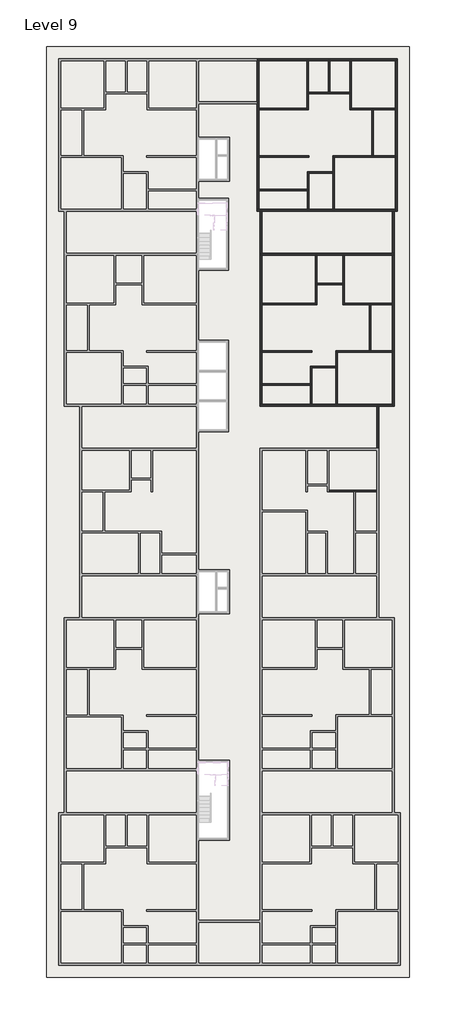
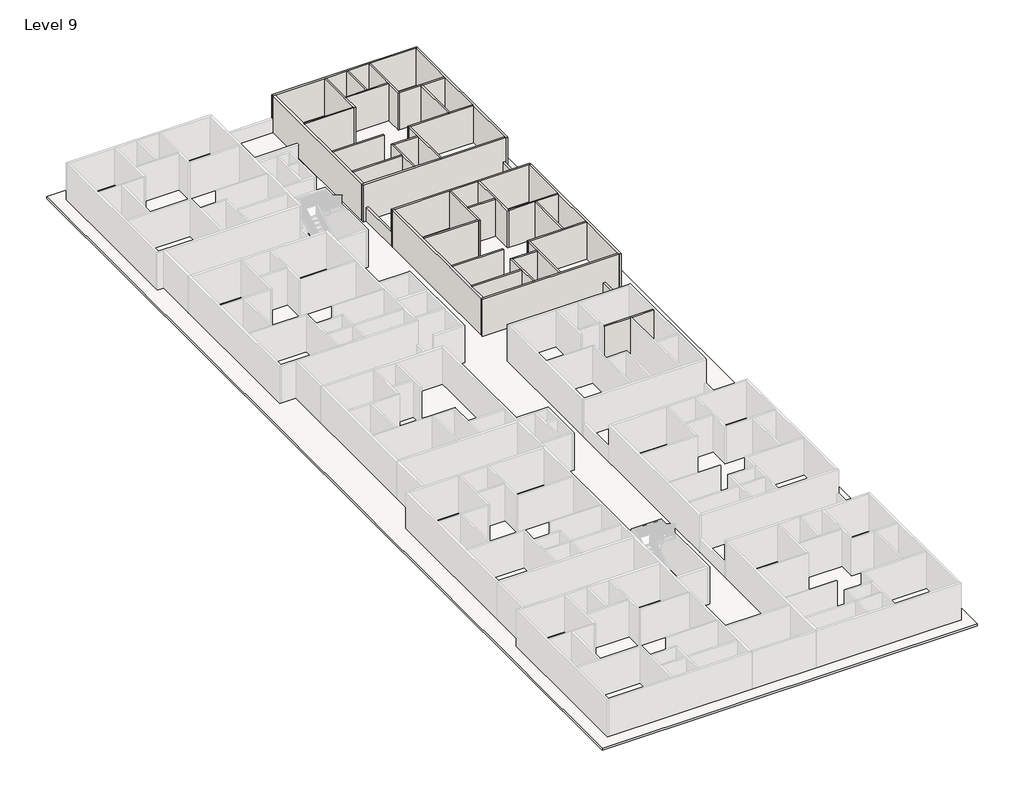
# One storey, part 4 of 8: 37 walls, 1 roof, 1 slab.
"""IFC4 building model written with IfcOpenShell, lengths in millimetres."""

from ifc_helpers import new_model, si_unit, frame, origin, place, context, project, spatial, polyline, outline, extrude, faceted_brep, element, save

model = new_model("IFC4")

# Units and contexts
model_context = context("Model", 3, world=origin())
ifc_project = project(units=[si_unit("LENGTHUNIT", "METRE", prefix="MILLI")], contexts=[model_context])

# Site, building, storey
site = spatial("IfcSite", under=ifc_project)
building = spatial("IfcBuilding", under=site)
storey = spatial("IfcBuildingStorey", under=building, Name="Level 9", Elevation=49618.6172466)

# Roof
placement = place(None, origin())
element("IfcRoof", 1, ObjectType="SLAB", at=placement, inside=storey, context=model_context, shape_type="SweptSolid", body=[
    extrude(outline(polyline([(-15237.9415084, -35021.5344126), (-15237.9415084, 36097.9216096), (12498.9443719, 36097.9216096), (12498.9443719, -35021.5344126), (-15237.9415084, -35021.5344126)]), holes=[polyline([(-3617.4415084, 29152.4900967), (-3617.4415084, 25799.6900967), (-1255.2415084, 25799.6900967), (-1255.2415084, 29152.4900967), (-3617.4415084, 29152.4900967)]), polyline([(-3617.4415084, 24490.1216096), (-3617.4415084, 19003.7216096), (-1331.4415084, 19003.7216096), (-1331.4415084, 24490.1216096), (-3617.4415084, 24490.1216096)]), polyline([(-3617.4415084, 13669.6303368), (-3617.4415084, 6659.2303368), (-1331.4415084, 6659.2303368), (-1331.4415084, 13669.6303368), (-3617.4415084, 13669.6303368)]), polyline([(-3617.4415084, -3882.2751812), (-3617.4415084, -7235.0751812), (-1255.2415084, -7235.0751812), (-1255.2415084, -3882.2751812), (-3617.4415084, -3882.2751812)]), polyline([(-3617.4415084, -18429.9851539), (-3617.4415084, -24525.9851539), (-1229.8415084, -24525.9851539), (-1229.8415084, -18429.9851539), (-3617.4415084, -18429.9851539)])]), frame((0.0, 0.0, 49618.6172466), z_axis=(0.0, 0.0, 1.0), x_axis=(1.0, 0.0, 0.0)), (0.0, 0.0, 1.0), 152.4),
])

# Slab
element("IfcSlab", 2, ObjectType="FLOOR", at=placement, inside=storey, context=model_context, shape_type="SweptSolid", body=[
    extrude(outline(polyline([(-14323.5415084, 35183.5216096), (11584.5443719, 35183.5216096), (11584.5443719, 23499.5216096), (11360.9214687, 23499.5216096), (11360.9214687, 8615.1216096), (10173.4714687, 8615.1216096), (10173.4714687, -7538.7344126), (11360.9214687, -7538.7344126), (11360.9214687, -22423.1344126), (11813.0584916, -22423.1344126), (11813.0584916, -34107.1344126), (11584.5443719, -34107.1344126), (-14323.5415084, -34107.1344126), (-14323.5415084, 35183.5216096)]), holes=[polyline([(-3617.4415084, 29152.4900967), (-3617.4415084, 25799.6900967), (-1255.2415084, 25799.6900967), (-1255.2415084, 29152.4900967), (-3617.4415084, 29152.4900967)]), polyline([(-3617.4415084, 24490.1216096), (-3617.4415084, 19003.7216096), (-1331.4415084, 19003.7216096), (-1331.4415084, 24490.1216096), (-3617.4415084, 24490.1216096)]), polyline([(-3617.4415084, 13669.6303368), (-3617.4415084, 6659.2303368), (-1331.4415084, 6659.2303368), (-1331.4415084, 13669.6303368), (-3617.4415084, 13669.6303368)]), polyline([(-3617.4415084, -3882.2751812), (-3617.4415084, -7235.0751812), (-1255.2415084, -7235.0751812), (-1255.2415084, -3882.2751812), (-3617.4415084, -3882.2751812)]), polyline([(-3617.4415084, -18429.9851539), (-3617.4415084, -24525.9851539), (-1229.8415084, -24525.9851539), (-1229.8415084, -18429.9851539), (-3617.4415084, -18429.9851539)])]), frame((0.0, 0.0, 49009.0172466), z_axis=(0.0, 0.0, 1.0), x_axis=(1.0, 0.0, 0.0)), (0.0, 0.0, 1.0), 609.6),
])

# Walls
element("IfcWall", 3, ObjectType="4.5\"", at=placement, inside=storey, context=model_context, shape_type="Brep", body=[
    faceted_brep([(6363.4714687, 2100.0216096, 49618.6172466), (8282.4584916, 2100.0216096, 49618.6172466), (8396.7584916, 2100.0216096, 49618.6172466), (10021.0714687, 2100.0216096, 49618.6172466), (10021.0714687, 2100.0216096, 52666.6172466), (8396.7584916, 2100.0216096, 52666.6172466), (8282.4584916, 2100.0216096, 52666.6172466), (6363.4714687, 2100.0216096, 52666.6172466), (6363.4714687, 2214.3216096, 49618.6172466), (6363.4714687, 2214.3216096, 52666.6172466), (10021.0714687, 2214.3216096, 52666.6172466), (10021.0714687, 2214.3216096, 49618.6172466)], [[[0, 1, 2, 3, 4, 5, 6, 7]], [[8, 9, 10, 11]], [[3, 2, 1, 0, 8, 11]], [[0, 7, 9, 8]], [[4, 3, 11, 10]], [[7, 6, 5, 4, 10, 9]]]),
])
element("IfcWall", 4, ObjectType="4.5\"", at=placement, inside=storey, context=model_context, shape_type="Brep", body=[
    faceted_brep([(5315.7214687, 20146.7216096, 49618.6172466), (5315.7214687, 16489.1216096, 49618.6172466), (5315.7214687, 16374.8216096, 49618.6172466), (5315.7214687, 16374.8216096, 52666.6172466), (5315.7214687, 16489.1216096, 52666.6172466), (5315.7214687, 20146.7216096, 52666.6172466), (5430.0214687, 20146.7216096, 49618.6172466), (5430.0214687, 20146.7216096, 52666.6172466), (5430.0214687, 18013.1216096, 52666.6172466), (5430.0214687, 17898.8216096, 52666.6172466), (5430.0214687, 16374.8216096, 52666.6172466), (5430.0214687, 16374.8216096, 49618.6172466), (5430.0214687, 17898.8216096, 49618.6172466), (5430.0214687, 18013.1216096, 49618.6172466)], [[[0, 1, 2, 3, 4, 5]], [[6, 7, 8, 9, 10, 11, 12, 13]], [[2, 1, 0, 6, 13, 12, 11]], [[0, 5, 7, 6]], [[3, 2, 11, 10]], [[5, 4, 3, 10, 9, 8, 7]]]),
])
element("IfcWall", 5, ObjectType="4.5\"", at=placement, inside=storey, context=model_context, shape_type="SweptSolid", body=[
    extrude(outline(polyline([(1259.3584916, 16489.1216096), (5315.7214687, 16489.1216096), (5315.7214687, 16374.8216096), (1259.3584916, 16374.8216096), (1259.3584916, 16489.1216096)])), frame((0.0, 0.0, 49618.6172466), z_axis=(0.0, 0.0, 1.0), x_axis=(1.0, 0.0, 0.0)), (0.0, 0.0, 1.0), 3048.0),
])
element("IfcWall", 6, ObjectType="4.5\"", at=placement, inside=storey, context=model_context, shape_type="SweptSolid", body=[
    extrude(outline(polyline([(7436.6214687, 17898.8216096), (5430.0214687, 17898.8216096), (5430.0214687, 18013.1216096), (7436.6214687, 18013.1216096), (7436.6214687, 17898.8216096)])), frame((0.0, 0.0, 49618.6172466), z_axis=(0.0, 0.0, 1.0), x_axis=(1.0, 0.0, 0.0)), (0.0, 0.0, 1.0), 3048.0),
])
element("IfcWall", 7, ObjectType="4.5\"", at=placement, inside=storey, context=model_context, shape_type="Brep", body=[
    faceted_brep([(7436.6214687, 20146.7216096, 49618.6172466), (7436.6214687, 18013.1216096, 49618.6172466), (7436.6214687, 17898.8216096, 49618.6172466), (7436.6214687, 16374.8216096, 49618.6172466), (7436.6214687, 16374.8216096, 52666.6172466), (7436.6214687, 17898.8216096, 52666.6172466), (7436.6214687, 18013.1216096, 52666.6172466), (7436.6214687, 20146.7216096, 52666.6172466), (7550.9214687, 20146.7216096, 49618.6172466), (7550.9214687, 20146.7216096, 52666.6172466), (7550.9214687, 16489.1216096, 52666.6172466), (7550.9214687, 16374.8216096, 52666.6172466), (7550.9214687, 16374.8216096, 49618.6172466), (7550.9214687, 16489.1216096, 49618.6172466)], [[[0, 1, 2, 3, 4, 5, 6, 7]], [[8, 9, 10, 11, 12, 13]], [[3, 2, 1, 0, 8, 13, 12]], [[0, 7, 9, 8]], [[4, 3, 12, 11]], [[7, 6, 5, 4, 11, 10, 9]]]),
])
element("IfcWall", 8, ObjectType="4.5\"", at=placement, inside=storey, context=model_context, shape_type="Brep", body=[
    faceted_brep([(7550.9214687, 16374.8216096, 49618.6172466), (9469.9084916, 16374.8216096, 49618.6172466), (9584.2084916, 16374.8216096, 49618.6172466), (11208.5214687, 16374.8216096, 49618.6172466), (11208.5214687, 16374.8216096, 52666.6172466), (9584.2084916, 16374.8216096, 52666.6172466), (9469.9084916, 16374.8216096, 52666.6172466), (7550.9214687, 16374.8216096, 52666.6172466), (7550.9214687, 16489.1216096, 49618.6172466), (7550.9214687, 16489.1216096, 52666.6172466), (11208.5214687, 16489.1216096, 52666.6172466), (11208.5214687, 16489.1216096, 49618.6172466)], [[[0, 1, 2, 3, 4, 5, 6, 7]], [[8, 9, 10, 11]], [[3, 2, 1, 0, 8, 11]], [[0, 7, 9, 8]], [[4, 3, 11, 10]], [[7, 6, 5, 4, 10, 9]]]),
])
element("IfcWall", 9, ObjectType="4.5\"", at=placement, inside=storey, context=model_context, shape_type="SweptSolid", body=[
    extrude(outline(polyline([(9469.9084916, 12869.6216096), (9469.9084916, 16374.8216096), (9584.2084916, 16374.8216096), (9584.2084916, 12869.6216096), (9469.9084916, 12869.6216096)])), frame((0.0, 0.0, 49618.6172466), z_axis=(0.0, 0.0, 1.0), x_axis=(1.0, 0.0, 0.0)), (0.0, 0.0, 1.0), 3048.0),
])
element("IfcWall", 10, ObjectType="4.5\"", at=placement, inside=storey, context=model_context, shape_type="Brep", body=[
    faceted_brep([(11208.5214687, 12869.6216096, 49618.6172466), (9584.2084916, 12869.6216096, 49618.6172466), (9469.9084916, 12869.6216096, 49618.6172466), (6885.4584916, 12869.6216096, 49618.6172466), (6885.4584916, 12869.6216096, 52666.6172466), (9469.9084916, 12869.6216096, 52666.6172466), (9584.2084916, 12869.6216096, 52666.6172466), (11208.5214687, 12869.6216096, 52666.6172466), (11208.5214687, 12755.3216096, 49618.6172466), (11208.5214687, 12755.3216096, 52666.6172466), (6999.7584916, 12755.3216096, 52666.6172466), (6885.4584916, 12755.3216096, 52666.6172466), (6885.4584916, 12755.3216096, 49618.6172466), (6999.7584916, 12755.3216096, 49618.6172466)], [[[0, 1, 2, 3, 4, 5, 6, 7]], [[8, 9, 10, 11, 12, 13]], [[3, 2, 1, 0, 8, 13, 12]], [[0, 7, 9, 8]], [[4, 3, 12, 11]], [[7, 6, 5, 4, 11, 10, 9]]]),
])
element("IfcWall", 11, ObjectType="4.5\"", at=placement, inside=storey, context=model_context, shape_type="Brep", body=[
    faceted_brep([(6885.4584916, 12755.3216096, 49618.6172466), (6885.4584916, 11663.1216096, 49618.6172466), (6885.4584916, 11548.8216096, 49618.6172466), (6885.4584916, 8767.5216096, 49618.6172466), (6885.4584916, 8767.5216096, 52666.6172466), (6885.4584916, 11548.8216096, 52666.6172466), (6885.4584916, 11663.1216096, 52666.6172466), (6885.4584916, 12755.3216096, 52666.6172466), (6999.7584916, 12755.3216096, 49618.6172466), (6999.7584916, 12755.3216096, 52666.6172466), (6999.7584916, 8767.5216096, 52666.6172466), (6999.7584916, 8767.5216096, 49618.6172466)], [[[0, 1, 2, 3, 4, 5, 6, 7]], [[8, 9, 10, 11]], [[3, 2, 1, 0, 8, 11]], [[0, 7, 9, 8]], [[4, 3, 11, 10]], [[7, 6, 5, 4, 10, 9]]]),
])
element("IfcWall", 12, ObjectType="4.5\"", at=placement, inside=storey, context=model_context, shape_type="Brep", body=[
    faceted_brep([(5056.6584916, 8767.5216096, 49618.6172466), (5056.6584916, 11548.8216096, 49618.6172466), (5056.6584916, 11663.1216096, 49618.6172466), (5056.6584916, 11663.1216096, 52666.6172466), (5056.6584916, 11548.8216096, 52666.6172466), (5056.6584916, 8767.5216096, 52666.6172466), (4942.3584916, 8767.5216096, 49618.6172466), (4942.3584916, 8767.5216096, 52666.6172466), (4942.3584916, 10215.3216096, 52666.6172466), (4942.3584916, 10329.6216096, 52666.6172466), (4942.3584916, 11663.1216096, 52666.6172466), (4942.3584916, 11663.1216096, 49618.6172466), (4942.3584916, 10329.6216096, 49618.6172466), (4942.3584916, 10215.3216096, 49618.6172466)], [[[0, 1, 2, 3, 4, 5]], [[6, 7, 8, 9, 10, 11, 12, 13]], [[2, 1, 0, 6, 13, 12, 11]], [[0, 5, 7, 6]], [[3, 2, 11, 10]], [[5, 4, 3, 10, 9, 8, 7]]]),
])
element("IfcWall", 13, ObjectType="4.5\"", at=placement, inside=storey, context=model_context, shape_type="SweptSolid", body=[
    extrude(outline(polyline([(6885.4584916, 11548.8216096), (5056.6584916, 11548.8216096), (5056.6584916, 11663.1216096), (6885.4584916, 11663.1216096), (6885.4584916, 11548.8216096)])), frame((0.0, 0.0, 49618.6172466), z_axis=(0.0, 0.0, 1.0), x_axis=(1.0, 0.0, 0.0)), (0.0, 0.0, 1.0), 3048.0),
])
element("IfcWall", 14, ObjectType="4.5\"", at=placement, inside=storey, context=model_context, shape_type="SweptSolid", body=[
    extrude(outline(polyline([(4942.3584916, 10215.3216096), (1259.3584916, 10215.3216096), (1259.3584916, 10329.6216096), (4942.3584916, 10329.6216096), (4942.3584916, 10215.3216096)])), frame((0.0, 0.0, 49618.6172466), z_axis=(0.0, 0.0, 1.0), x_axis=(1.0, 0.0, 0.0)), (0.0, 0.0, 1.0), 3048.0),
])
element("IfcWall", 15, ObjectType="4.5\"", at=placement, inside=storey, context=model_context, shape_type="SweptSolid", body=[
    extrude(outline(polyline([(5056.6584916, 12755.3216096), (1259.3584916, 12755.3216096), (1259.3584916, 12869.6216096), (5056.6584916, 12869.6216096), (5056.6584916, 12755.3216096)])), frame((0.0, 0.0, 49618.6172466), z_axis=(0.0, 0.0, 1.0), x_axis=(1.0, 0.0, 0.0)), (0.0, 0.0, 1.0), 3048.0),
])
element("IfcWall", 16, ObjectType="4.5\"", at=placement, inside=storey, context=model_context, shape_type="Brep", body=[
    faceted_brep([(4688.4443719, 35031.1216096, 49618.6172466), (4688.4443719, 31373.5216096, 49618.6172466), (4688.4443719, 31259.2216096, 49618.6172466), (4688.4443719, 31259.2216096, 52666.6172466), (4688.4443719, 31373.5216096, 52666.6172466), (4688.4443719, 35031.1216096, 52666.6172466), (4802.7443719, 35031.1216096, 49618.6172466), (4802.7443719, 35031.1216096, 52666.6172466), (4802.7443719, 32592.7216096, 52666.6172466), (4802.7443719, 32478.4216096, 52666.6172466), (4802.7443719, 31259.2216096, 52666.6172466), (4802.7443719, 31259.2216096, 49618.6172466), (4802.7443719, 32478.4216096, 49618.6172466), (4802.7443719, 32592.7216096, 49618.6172466)], [[[0, 1, 2, 3, 4, 5]], [[6, 7, 8, 9, 10, 11, 12, 13]], [[2, 1, 0, 6, 13, 12, 11]], [[0, 5, 7, 6]], [[3, 2, 11, 10]], [[5, 4, 3, 10, 9, 8, 7]]]),
])
element("IfcWall", 17, ObjectType="4.5\"", at=placement, inside=storey, context=model_context, shape_type="SweptSolid", body=[
    extrude(outline(polyline([(1030.8443719, 31373.5216096), (4688.4443719, 31373.5216096), (4688.4443719, 31259.2216096), (1030.8443719, 31259.2216096), (1030.8443719, 31373.5216096)])), frame((0.0, 0.0, 49618.6172466), z_axis=(0.0, 0.0, 1.0), x_axis=(1.0, 0.0, 0.0)), (0.0, 0.0, 1.0), 3048.0),
])
element("IfcWall", 18, ObjectType="4.5\"", at=placement, inside=storey, context=model_context, shape_type="Brep", body=[
    faceted_brep([(4802.7443719, 32478.4216096, 49618.6172466), (7965.0443719, 32478.4216096, 49618.6172466), (7965.0443719, 32478.4216096, 52666.6172466), (4802.7443719, 32478.4216096, 52666.6172466), (4802.7443719, 32592.7216096, 49618.6172466), (4802.7443719, 32592.7216096, 52666.6172466), (6326.7443719, 32592.7216096, 52666.6172466), (6441.0443719, 32592.7216096, 52666.6172466), (7965.0443719, 32592.7216096, 52666.6172466), (7965.0443719, 32592.7216096, 49618.6172466), (6441.0443719, 32592.7216096, 49618.6172466), (6326.7443719, 32592.7216096, 49618.6172466)], [[[0, 1, 2, 3]], [[4, 5, 6, 7, 8, 9, 10, 11]], [[1, 0, 4, 11, 10, 9]], [[0, 3, 5, 4]], [[2, 1, 9, 8]], [[3, 2, 8, 7, 6, 5]]]),
])
element("IfcWall", 19, ObjectType="4.5\"", at=placement, inside=storey, context=model_context, shape_type="SweptSolid", body=[
    extrude(outline(polyline([(6326.7443719, 32592.7216096), (6326.7443719, 35031.1216096), (6441.0443719, 35031.1216096), (6441.0443719, 32592.7216096), (6326.7443719, 32592.7216096)])), frame((0.0, 0.0, 49618.6172466), z_axis=(0.0, 0.0, 1.0), x_axis=(1.0, 0.0, 0.0)), (0.0, 0.0, 1.0), 3048.0),
])
element("IfcWall", 20, ObjectType="4.5\"", at=placement, inside=storey, context=model_context, shape_type="Brep", body=[
    faceted_brep([(7965.0443719, 35031.1216096, 49618.6172466), (7965.0443719, 32592.7216096, 49618.6172466), (7965.0443719, 32478.4216096, 49618.6172466), (7965.0443719, 31259.2216096, 49618.6172466), (7965.0443719, 31259.2216096, 52666.6172466), (7965.0443719, 32478.4216096, 52666.6172466), (7965.0443719, 32592.7216096, 52666.6172466), (7965.0443719, 35031.1216096, 52666.6172466), (8079.3443719, 35031.1216096, 49618.6172466), (8079.3443719, 35031.1216096, 52666.6172466), (8079.3443719, 31373.5216096, 52666.6172466), (8079.3443719, 31259.2216096, 52666.6172466), (8079.3443719, 31259.2216096, 49618.6172466), (8079.3443719, 31373.5216096, 49618.6172466)], [[[0, 1, 2, 3, 4, 5, 6, 7]], [[8, 9, 10, 11, 12, 13]], [[3, 2, 1, 0, 8, 13, 12]], [[0, 7, 9, 8]], [[4, 3, 12, 11]], [[7, 6, 5, 4, 11, 10, 9]]]),
])
element("IfcWall", 21, ObjectType="4.5\"", at=placement, inside=storey, context=model_context, shape_type="Brep", body=[
    faceted_brep([(8079.3443719, 31259.2216096, 49618.6172466), (9641.4443719, 31259.2216096, 49618.6172466), (9755.7443719, 31259.2216096, 49618.6172466), (11432.1443719, 31259.2216096, 49618.6172466), (11432.1443719, 31259.2216096, 52666.6172466), (9755.7443719, 31259.2216096, 52666.6172466), (9641.4443719, 31259.2216096, 52666.6172466), (8079.3443719, 31259.2216096, 52666.6172466), (8079.3443719, 31373.5216096, 49618.6172466), (8079.3443719, 31373.5216096, 52666.6172466), (11432.1443719, 31373.5216096, 52666.6172466), (11432.1443719, 31373.5216096, 49618.6172466)], [[[0, 1, 2, 3, 4, 5, 6, 7]], [[8, 9, 10, 11]], [[3, 2, 1, 0, 8, 11]], [[0, 7, 9, 8]], [[4, 3, 11, 10]], [[7, 6, 5, 4, 10, 9]]]),
])
element("IfcWall", 22, ObjectType="4.5\"", at=placement, inside=storey, context=model_context, shape_type="SweptSolid", body=[
    extrude(outline(polyline([(9641.4443719, 27754.0216096), (9641.4443719, 31259.2216096), (9755.7443719, 31259.2216096), (9755.7443719, 27754.0216096), (9641.4443719, 27754.0216096)])), frame((0.0, 0.0, 49618.6172466), z_axis=(0.0, 0.0, 1.0), x_axis=(1.0, 0.0, 0.0)), (0.0, 0.0, 1.0), 3048.0),
])
element("IfcWall", 23, ObjectType="4.5\"", at=placement, inside=storey, context=model_context, shape_type="Brep", body=[
    faceted_brep([(11432.1443719, 27754.0216096, 49618.6172466), (9755.7443719, 27754.0216096, 49618.6172466), (9641.4443719, 27754.0216096, 49618.6172466), (6656.9443719, 27754.0216096, 49618.6172466), (6656.9443719, 27754.0216096, 52666.6172466), (9641.4443719, 27754.0216096, 52666.6172466), (9755.7443719, 27754.0216096, 52666.6172466), (11432.1443719, 27754.0216096, 52666.6172466), (11432.1443719, 27639.7216096, 49618.6172466), (11432.1443719, 27639.7216096, 52666.6172466), (6771.2443719, 27639.7216096, 52666.6172466), (6656.9443719, 27639.7216096, 52666.6172466), (6656.9443719, 27639.7216096, 49618.6172466), (6771.2443719, 27639.7216096, 49618.6172466)], [[[0, 1, 2, 3, 4, 5, 6, 7]], [[8, 9, 10, 11, 12, 13]], [[3, 2, 1, 0, 8, 13, 12]], [[0, 7, 9, 8]], [[4, 3, 12, 11]], [[7, 6, 5, 4, 11, 10, 9]]]),
])
element("IfcWall", 24, ObjectType="4.5\"", at=placement, inside=storey, context=model_context, shape_type="Brep", body=[
    faceted_brep([(6656.9443719, 27639.7216096, 49618.6172466), (6656.9443719, 26547.5216096, 49618.6172466), (6656.9443719, 26433.2216096, 49618.6172466), (6656.9443719, 23651.9216096, 49618.6172466), (6656.9443719, 23651.9216096, 52666.6172466), (6656.9443719, 26433.2216096, 52666.6172466), (6656.9443719, 26547.5216096, 52666.6172466), (6656.9443719, 27639.7216096, 52666.6172466), (6771.2443719, 27639.7216096, 49618.6172466), (6771.2443719, 27639.7216096, 52666.6172466), (6771.2443719, 23651.9216096, 52666.6172466), (6771.2443719, 23651.9216096, 49618.6172466)], [[[0, 1, 2, 3, 4, 5, 6, 7]], [[8, 9, 10, 11]], [[3, 2, 1, 0, 8, 11]], [[0, 7, 9, 8]], [[4, 3, 11, 10]], [[7, 6, 5, 4, 10, 9]]]),
])
element("IfcWall", 25, ObjectType="4.5\"", at=placement, inside=storey, context=model_context, shape_type="SweptSolid", body=[
    extrude(outline(polyline([(4713.8443719, 25099.7216096), (1030.8443719, 25099.7216096), (1030.8443719, 25214.0216096), (4713.8443719, 25214.0216096), (4713.8443719, 25099.7216096)])), frame((0.0, 0.0, 49618.6172466), z_axis=(0.0, 0.0, 1.0), x_axis=(1.0, 0.0, 0.0)), (0.0, 0.0, 1.0), 3048.0),
])
element("IfcWall", 26, ObjectType="4.5\"", at=placement, inside=storey, context=model_context, shape_type="Brep", body=[
    faceted_brep([(4828.1443719, 23651.9216096, 49618.6172466), (4828.1443719, 26433.2216096, 49618.6172466), (4828.1443719, 26547.5216096, 49618.6172466), (4828.1443719, 26547.5216096, 52666.6172466), (4828.1443719, 26433.2216096, 52666.6172466), (4828.1443719, 23651.9216096, 52666.6172466), (4713.8443719, 23651.9216096, 49618.6172466), (4713.8443719, 23651.9216096, 52666.6172466), (4713.8443719, 25099.7216096, 52666.6172466), (4713.8443719, 25214.0216096, 52666.6172466), (4713.8443719, 26547.5216096, 52666.6172466), (4713.8443719, 26547.5216096, 49618.6172466), (4713.8443719, 25214.0216096, 49618.6172466), (4713.8443719, 25099.7216096, 49618.6172466)], [[[0, 1, 2, 3, 4, 5]], [[6, 7, 8, 9, 10, 11, 12, 13]], [[2, 1, 0, 6, 13, 12, 11]], [[0, 5, 7, 6]], [[3, 2, 11, 10]], [[5, 4, 3, 10, 9, 8, 7]]]),
])
element("IfcWall", 27, ObjectType="4.5\"", at=placement, inside=storey, context=model_context, shape_type="SweptSolid", body=[
    extrude(outline(polyline([(6656.9443719, 26433.2216096), (4828.1443719, 26433.2216096), (4828.1443719, 26547.5216096), (6656.9443719, 26547.5216096), (6656.9443719, 26433.2216096)])), frame((0.0, 0.0, 49618.6172466), z_axis=(0.0, 0.0, 1.0), x_axis=(1.0, 0.0, 0.0)), (0.0, 0.0, 1.0), 3048.0),
])
element("IfcWall", 28, ObjectType="4.5\"", at=placement, inside=storey, context=model_context, shape_type="SweptSolid", body=[
    extrude(outline(polyline([(4828.1443719, 27639.7216096), (1030.8443719, 27639.7216096), (1030.8443719, 27754.0216096), (4828.1443719, 27754.0216096), (4828.1443719, 27639.7216096)])), frame((0.0, 0.0, 49618.6172466), z_axis=(0.0, 0.0, 1.0), x_axis=(1.0, 0.0, 0.0)), (0.0, 0.0, 1.0), 3048.0),
])
element("IfcWall", 29, ObjectType="6\"", at=placement, inside=storey, context=model_context, shape_type="Brep", body=[
    faceted_brep([(1106.9584916, 20146.7216096, 52666.6172466), (1106.9584916, 20146.7216096, 49618.6172466), (1259.3584916, 20146.7216096, 49618.6172466), (5315.7214687, 20146.7216096, 49618.6172466), (5430.0214687, 20146.7216096, 49618.6172466), (7436.6214687, 20146.7216096, 49618.6172466), (7550.9214687, 20146.7216096, 49618.6172466), (11208.5214687, 20146.7216096, 49618.6172466), (11360.9214687, 20146.7216096, 49618.6172466), (11360.9214687, 20146.7216096, 52666.6172466), (11208.5214687, 20146.7216096, 52666.6172466), (7550.9214687, 20146.7216096, 52666.6172466), (7436.6214687, 20146.7216096, 52666.6172466), (5430.0214687, 20146.7216096, 52666.6172466), (5315.7214687, 20146.7216096, 52666.6172466), (1259.3584916, 20146.7216096, 52666.6172466), (1106.9584916, 20299.1216096, 49618.6172466), (1106.9584916, 20299.1216096, 50837.8172466), (1106.9584916, 20299.1216096, 52666.6172466), (11360.9214687, 20299.1216096, 52666.6172466), (11360.9214687, 20299.1216096, 50837.8172466), (11360.9214687, 20299.1216096, 49618.6172466), (11208.5214687, 20299.1216096, 49618.6172466), (1259.3584916, 20299.1216096, 49618.6172466)], [[[0, 1, 2, 3, 4, 5, 6, 7, 8, 9, 10, 11, 12, 13, 14, 15]], [[16, 17, 18, 19, 20, 21, 22, 23]], [[8, 7, 6, 5, 4, 3, 2, 1, 16, 23, 22, 21]], [[0, 18, 17, 16, 1]], [[8, 21, 20, 19, 9]], [[0, 15, 14, 13, 12, 11, 10, 9, 19, 18]]]),
])
element("IfcWall", 30, ObjectType="6\"", at=placement, inside=storey, context=model_context, shape_type="Brep", body=[
    faceted_brep([(11208.5214687, 20146.7216096, 52666.6172466), (11208.5214687, 20146.7216096, 49618.6172466), (11208.5214687, 16489.1216096, 49618.6172466), (11208.5214687, 16374.8216096, 49618.6172466), (11208.5214687, 12869.6216096, 49618.6172466), (11208.5214687, 12755.3216096, 49618.6172466), (11208.5214687, 8767.5216096, 49618.6172466), (11208.5214687, 8615.1216096, 49618.6172466), (11208.5214687, 8615.1216096, 52666.6172466), (11208.5214687, 8767.5216096, 52666.6172466), (11208.5214687, 12755.3216096, 52666.6172466), (11208.5214687, 12869.6216096, 52666.6172466), (11208.5214687, 16374.8216096, 52666.6172466), (11208.5214687, 16489.1216096, 52666.6172466), (11360.9214687, 20146.7216096, 49618.6172466), (11360.9214687, 20146.7216096, 52666.6172466), (11360.9214687, 8615.1216096, 52666.6172466), (11360.9214687, 8615.1216096, 49618.6172466)], [[[0, 1, 2, 3, 4, 5, 6, 7, 8, 9, 10, 11, 12, 13]], [[14, 15, 16, 17]], [[7, 6, 5, 4, 3, 2, 1, 14, 17]], [[8, 7, 17, 16]], [[0, 15, 14, 1]], [[0, 13, 12, 11, 10, 9, 8, 16, 15]]]),
])
element("IfcWall", 31, ObjectType="6\"", at=placement, inside=storey, context=model_context, shape_type="Brep", body=[
    faceted_brep([(11208.5214687, 8767.5216096, 49618.6172466), (6999.7584916, 8767.5216096, 49618.6172466), (6885.4584916, 8767.5216096, 49618.6172466), (5056.6584916, 8767.5216096, 49618.6172466), (4942.3584916, 8767.5216096, 49618.6172466), (1259.3584916, 8767.5216096, 49618.6172466), (1106.9584916, 8767.5216096, 49618.6172466), (1106.9584916, 8767.5216096, 52666.6172466), (1259.3584916, 8767.5216096, 52666.6172466), (4942.3584916, 8767.5216096, 52666.6172466), (5056.6584916, 8767.5216096, 52666.6172466), (6885.4584916, 8767.5216096, 52666.6172466), (6999.7584916, 8767.5216096, 52666.6172466), (11208.5214687, 8767.5216096, 52666.6172466), (11208.5214687, 8615.1216096, 49618.6172466), (11208.5214687, 8615.1216096, 52666.6172466), (1106.9584916, 8615.1216096, 52666.6172466), (1106.9584916, 8615.1216096, 49618.6172466), (10021.0714687, 8615.1216096, 49618.6172466), (10173.4714687, 8615.1216096, 49618.6172466)], [[[0, 1, 2, 3, 4, 5, 6, 7, 8, 9, 10, 11, 12, 13]], [[14, 15, 16, 17, 18, 19]], [[6, 5, 4, 3, 2, 1, 0, 14, 19, 18, 17]], [[0, 13, 15, 14]], [[7, 6, 17, 16]], [[13, 12, 11, 10, 9, 8, 7, 16, 15]]]),
])
element("IfcWall", 32, ObjectType="6\"", at=placement, inside=storey, context=model_context, shape_type="Brep", body=[
    faceted_brep([(1259.3584916, 8767.5216096, 49618.6172466), (1259.3584916, 10215.3216096, 49618.6172466), (1259.3584916, 10329.6216096, 49618.6172466), (1259.3584916, 12755.3216096, 49618.6172466), (1259.3584916, 12869.6216096, 49618.6172466), (1259.3584916, 16374.8216096, 49618.6172466), (1259.3584916, 16489.1216096, 49618.6172466), (1259.3584916, 20146.7216096, 49618.6172466), (1259.3584916, 20146.7216096, 52666.6172466), (1259.3584916, 16489.1216096, 52666.6172466), (1259.3584916, 16374.8216096, 52666.6172466), (1259.3584916, 12869.6216096, 52666.6172466), (1259.3584916, 12755.3216096, 52666.6172466), (1259.3584916, 10329.6216096, 52666.6172466), (1259.3584916, 10215.3216096, 52666.6172466), (1259.3584916, 8767.5216096, 52666.6172466), (1106.9584916, 8767.5216096, 49618.6172466), (1106.9584916, 8767.5216096, 52666.6172466), (1106.9584916, 20146.7216096, 52666.6172466), (1106.9584916, 20146.7216096, 49618.6172466)], [[[0, 1, 2, 3, 4, 5, 6, 7, 8, 9, 10, 11, 12, 13, 14, 15]], [[16, 17, 18, 19]], [[7, 6, 5, 4, 3, 2, 1, 0, 16, 19]], [[0, 15, 17, 16]], [[7, 19, 18, 8]], [[15, 14, 13, 12, 11, 10, 9, 8, 18, 17]]]),
])
element("IfcWall", 33, ObjectType="6\"", at=placement, inside=storey, context=model_context, shape_type="Brep", body=[
    faceted_brep([(878.4443719, 35031.1216096, 52666.6172466), (878.4443719, 35031.1216096, 49618.6172466), (1030.8443719, 35031.1216096, 49618.6172466), (4688.4443719, 35031.1216096, 49618.6172466), (4802.7443719, 35031.1216096, 49618.6172466), (6326.7443719, 35031.1216096, 49618.6172466), (6441.0443719, 35031.1216096, 49618.6172466), (7965.0443719, 35031.1216096, 49618.6172466), (8079.3443719, 35031.1216096, 49618.6172466), (11432.1443719, 35031.1216096, 49618.6172466), (11584.5443719, 35031.1216096, 49618.6172466), (11584.5443719, 35031.1216096, 52666.6172466), (11432.1443719, 35031.1216096, 52666.6172466), (8079.3443719, 35031.1216096, 52666.6172466), (7965.0443719, 35031.1216096, 52666.6172466), (6441.0443719, 35031.1216096, 52666.6172466), (6326.7443719, 35031.1216096, 52666.6172466), (4802.7443719, 35031.1216096, 52666.6172466), (4688.4443719, 35031.1216096, 52666.6172466), (1030.8443719, 35031.1216096, 52666.6172466), (878.4443719, 35183.5216096, 49618.6172466), (878.4443719, 35183.5216096, 52666.6172466), (11584.5443719, 35183.5216096, 52666.6172466), (11584.5443719, 35183.5216096, 49618.6172466)], [[[0, 1, 2, 3, 4, 5, 6, 7, 8, 9, 10, 11, 12, 13, 14, 15, 16, 17, 18, 19]], [[20, 21, 22, 23]], [[10, 9, 8, 7, 6, 5, 4, 3, 2, 1, 20, 23]], [[11, 10, 23, 22]], [[0, 21, 20, 1]], [[0, 19, 18, 17, 16, 15, 14, 13, 12, 11, 22, 21]]]),
])
element("IfcWall", 34, ObjectType="6\"", at=placement, inside=storey, context=model_context, shape_type="Brep", body=[
    faceted_brep([(11432.1443719, 35031.1216096, 49618.6172466), (11432.1443719, 31373.5216096, 49618.6172466), (11432.1443719, 31259.2216096, 49618.6172466), (11432.1443719, 27754.0216096, 49618.6172466), (11432.1443719, 27639.7216096, 49618.6172466), (11432.1443719, 23651.9216096, 49618.6172466), (11432.1443719, 23499.5216096, 49618.6172466), (11432.1443719, 23499.5216096, 52666.6172466), (11432.1443719, 23651.9216096, 52666.6172466), (11432.1443719, 27639.7216096, 52666.6172466), (11432.1443719, 27754.0216096, 52666.6172466), (11432.1443719, 31259.2216096, 52666.6172466), (11432.1443719, 31373.5216096, 52666.6172466), (11432.1443719, 35031.1216096, 52666.6172466), (11584.5443719, 35031.1216096, 49618.6172466), (11584.5443719, 35031.1216096, 52666.6172466), (11584.5443719, 23499.5216096, 52666.6172466), (11584.5443719, 23499.5216096, 49618.6172466)], [[[0, 1, 2, 3, 4, 5, 6, 7, 8, 9, 10, 11, 12, 13]], [[14, 15, 16, 17]], [[6, 5, 4, 3, 2, 1, 0, 14, 17]], [[0, 13, 15, 14]], [[7, 6, 17, 16]], [[13, 12, 11, 10, 9, 8, 7, 16, 15]]]),
])
element("IfcWall", 35, ObjectType="6\"", at=placement, inside=storey, context=model_context, shape_type="Brep", body=[
    faceted_brep([(11432.1443719, 23651.9216096, 49618.6172466), (6771.2443719, 23651.9216096, 49618.6172466), (6656.9443719, 23651.9216096, 49618.6172466), (4828.1443719, 23651.9216096, 49618.6172466), (4713.8443719, 23651.9216096, 49618.6172466), (1030.8443719, 23651.9216096, 49618.6172466), (878.4443719, 23651.9216096, 49618.6172466), (878.4443719, 23651.9216096, 52666.6172466), (1030.8443719, 23651.9216096, 52666.6172466), (4713.8443719, 23651.9216096, 52666.6172466), (4828.1443719, 23651.9216096, 52666.6172466), (6656.9443719, 23651.9216096, 52666.6172466), (6771.2443719, 23651.9216096, 52666.6172466), (11432.1443719, 23651.9216096, 52666.6172466), (11432.1443719, 23499.5216096, 49618.6172466), (11432.1443719, 23499.5216096, 52666.6172466), (878.4443719, 23499.5216096, 52666.6172466), (878.4443719, 23499.5216096, 49618.6172466), (1106.9584916, 23499.5216096, 49618.6172466), (1259.3584916, 23499.5216096, 49618.6172466), (11208.5214687, 23499.5216096, 49618.6172466), (11360.9214687, 23499.5216096, 49618.6172466)], [[[0, 1, 2, 3, 4, 5, 6, 7, 8, 9, 10, 11, 12, 13]], [[14, 15, 16, 17, 18, 19, 20, 21]], [[6, 5, 4, 3, 2, 1, 0, 14, 21, 20, 19, 18, 17]], [[0, 13, 15, 14]], [[7, 6, 17, 16]], [[13, 12, 11, 10, 9, 8, 7, 16, 15]]]),
])
element("IfcWall", 36, ObjectType="6\"", at=placement, inside=storey, context=model_context, shape_type="Brep", body=[
    faceted_brep([(1030.8443719, 23651.9216096, 49618.6172466), (1030.8443719, 25099.7216096, 49618.6172466), (1030.8443719, 25214.0216096, 49618.6172466), (1030.8443719, 27639.7216096, 49618.6172466), (1030.8443719, 27754.0216096, 49618.6172466), (1030.8443719, 31259.2216096, 49618.6172466), (1030.8443719, 31373.5216096, 49618.6172466), (1030.8443719, 35031.1216096, 49618.6172466), (1030.8443719, 35031.1216096, 52666.6172466), (1030.8443719, 31373.5216096, 52666.6172466), (1030.8443719, 31259.2216096, 52666.6172466), (1030.8443719, 27754.0216096, 52666.6172466), (1030.8443719, 27639.7216096, 52666.6172466), (1030.8443719, 25214.0216096, 52666.6172466), (1030.8443719, 25099.7216096, 52666.6172466), (1030.8443719, 23651.9216096, 52666.6172466), (878.4443719, 23651.9216096, 49618.6172466), (878.4443719, 23651.9216096, 52666.6172466), (878.4443719, 35031.1216096, 52666.6172466), (878.4443719, 35031.1216096, 49618.6172466), (878.4443719, 31897.3197155, 49618.6172466), (878.4443719, 31744.9197155, 49618.6172466)], [[[0, 1, 2, 3, 4, 5, 6, 7, 8, 9, 10, 11, 12, 13, 14, 15]], [[16, 17, 18, 19, 20, 21]], [[7, 6, 5, 4, 3, 2, 1, 0, 16, 21, 20, 19]], [[0, 15, 17, 16]], [[7, 19, 18, 8]], [[15, 14, 13, 12, 11, 10, 9, 8, 18, 17]]]),
])
element("IfcWall", 37, ObjectType="6\" 2", at=placement, inside=storey, context=model_context, shape_type="SweptSolid", body=[
    extrude(outline(polyline([(1106.9584916, 20299.1216096), (1106.9584916, 23499.5216096), (1259.3584916, 23499.5216096), (1259.3584916, 20299.1216096), (1106.9584916, 20299.1216096)])), frame((0.0, 0.0, 49618.6172466), z_axis=(0.0, 0.0, 1.0), x_axis=(1.0, 0.0, 0.0)), (0.0, 0.0, 1.0), 1219.2),
])
element("IfcWall", 38, ObjectType="6\" 2", at=placement, inside=storey, context=model_context, shape_type="SweptSolid", body=[
    extrude(outline(polyline([(11208.5214687, 20299.1216096), (11208.5214687, 23499.5216096), (11360.9214687, 23499.5216096), (11360.9214687, 20299.1216096), (11208.5214687, 20299.1216096)])), frame((0.0, 0.0, 49618.6172466), z_axis=(0.0, 0.0, 1.0), x_axis=(1.0, 0.0, 0.0)), (0.0, 0.0, 1.0), 1219.2),
])
element("IfcWall", 39, ObjectType="6\" 2", at=placement, inside=storey, context=model_context, shape_type="SweptSolid", body=[
    extrude(outline(polyline([(10021.0714687, 5414.7216096), (10021.0714687, 8615.1216096), (10173.4714687, 8615.1216096), (10173.4714687, 5414.7216096), (10021.0714687, 5414.7216096)])), frame((0.0, 0.0, 49618.6172466), z_axis=(0.0, 0.0, 1.0), x_axis=(1.0, 0.0, 0.0)), (0.0, 0.0, 1.0), 1219.2),
])

save(model, "model.ifc")

# Revit data of these elements
# Type "SLAB"
#   Assembly Code = "B1020"
#   Layers, outside or top first: 0' - 6" "Damp-proofing" (function 1)
# Type "FLOOR"
#   Assembly Code = "B1010"
#   Function = 0
#   Layers, outside or top first: 2' - 0" "Tile, Porcelain, 4in" (function 1)
# Type "4.5\""
#   Assembly Code = "B2010"
#   Layers, outside or top first: 0' - 4 1/2" "WALLS" (function 1)
# Type "6\""
#   Assembly Code = "B2010"
#   Layers, outside or top first: 0' - 6" "WALLS" (function 1)
# Type "6\" 2"
#   Assembly Code = "B2010"
#   Layers, outside or top first: 0' - 6" "4'" (function 1)
# Element 1 (IfcRoof, "SLAB")
#   built-in parameter 1001705 = 163.291 (stored number, unit not read)
#   built-in parameter 1001710 = 33615
#   Phase Created = New Construction
#   Materials on its faces: "Damp-proofing"
# Element 2 (IfcSlab, "FLOOR")
#   built-in parameter 1001955 = 3.14159 (stored number, unit not read)
#   Height Offset From Level = 0' - 0"
#   Phase Created = New Construction
#   Materials on its faces: "Tile, Porcelain, 4in"
# Elements 3, 4, 5, 6, 7, 8, 9, 10, 11, 12, 13, 14, 15, 16, 17, 18, 19, 20, 21, 22, 23, 24, 25, 26, 27, 28 (IfcWall, "4.5\"")
#   Top Offset = 0' - 0"
#   Base Offset = 0' - 0"
#   Unconnected Height = 10' - 0"
#   wall height = 10' - 0"
#   Phase Created = New Construction
#   Base Constraint = Level 9
#   Materials on its faces: "WALLS"
# Elements 29, 30, 31, 32, 33, 34, 35, 36 (IfcWall, "6\"")
#   Top Offset = 0' - 0"
#   Base Offset = 0' - 0"
#   Unconnected Height = 10' - 0"
#   wall height = 10' - 0"
#   Phase Created = New Construction
#   Base Constraint = Level 9
#   Materials on its faces: "WALLS"
# Elements 37, 38, 39 (IfcWall, "6\" 2")
#   Top Offset = 0' - 0"
#   Base Offset = 0' - 0"
#   Unconnected Height = 4' - 0"
#   wall height = 4' - 0"
#   Phase Created = New Construction
#   Base Constraint = Level 9
#   Materials on its faces: "4'"
# Materials
#   "Damp-proofing": class "Generic", colour RGB 127 127 127, transparency 0, Description = "Damp-proofing", Cost = 0
#   "Tile, Porcelain, 4in": class "Generic", colour RGB 89 87 158, transparency 0, Description = "Porcelain tile, 4\", white", Cost = 0
#   "WALLS": class "Generic", colour RGB 120 120 120, transparency 0, Cost = 0
#   "4'": class "Generic", colour RGB 120 120 120, transparency 0, Cost = 0
